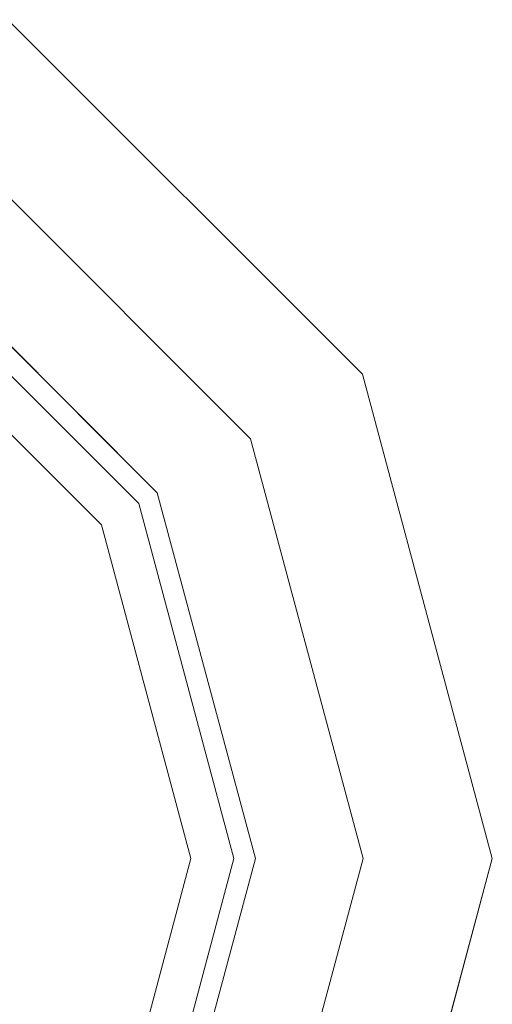
# Model space of a CAD drawing. Units: inches. Extents: x 375 to 1122, y 27 to 1069.
# Tile 45 of 155: x 715.392 to 718.094, y 302.255 to 307.886. Entities that reach past the tile are written whole.
import ezdxf

# ---------------------------------------------------------------- set-up
doc = ezdxf.new("R2010")
doc.units = ezdxf.units.IN
doc.layers.add('Furniture', color=30, linetype='Continuous', lineweight=18)

# ---------------------------------------------------------------- blocks, each defined once
blk = doc.blocks.new('A$C403C54AD')
at = {"linetype": 'ByBlock'}
for points, invisible_edges in [([(1.0802, 0.82864, -0.00874), (1.0802, 0.81017, -0.00874), (1.02018, 0.79408, -0.00874), (1.01094, 0.81008, -0.00874)], 5), ([(1.0802, 0.79478, -0.02259), (1.0802, 0.82864, -0.01335), (1.01094, 0.81008, -0.01335), (1.02787, 0.78075, -0.02259)], 5), ([(1.14947, 0.81008, -0.00874), (1.14023, 0.79408, -0.00874), (1.0802, 0.81017, -0.00874), (1.0802, 0.82864, -0.00874)], 5), ([(1.13254, 0.78075, -0.02259), (1.14947, 0.81008, -0.01335), (1.0802, 0.82864, -0.01335), (1.0802, 0.79478, -0.02259)], 5), ([(1.01094, 0.81008, -0.00874), (1.02018, 0.79408, -0.00874), (0.97623, 0.75014, -0.00874), (0.96024, 0.75938, -0.00874)], 5), ([(1.02787, 0.78075, -0.02259), (1.01094, 0.81008, -0.01335), (0.96024, 0.75938, -0.01335), (0.98956, 0.74244, -0.02259)], 5), ([(1.0802, 0.81017, -0.00874), (1.0802, 0.7917, -0.01489), (1.02941, 0.77809, -0.01489), (1.02018, 0.79408, -0.00874)], 5), ([(1.14023, 0.79408, -0.00874), (1.131, 0.77809, -0.01489), (1.0802, 0.7917, -0.01489), (1.0802, 0.81017, -0.00874)], 5), ([(1.02018, 0.79408, -0.00874), (1.02941, 0.77809, -0.01489), (0.99223, 0.74091, -0.01489), (0.97623, 0.75014, -0.00874)], 5), ([(1.0802, 0.78554, -0.03183), (1.0802, 0.79478, -0.02259), (1.02787, 0.78075, -0.02259), (1.03249, 0.77276, -0.03183)], 5), ([(1.12792, 0.77276, -0.03183), (1.13254, 0.78075, -0.02259), (1.0802, 0.79478, -0.02259), (1.0802, 0.78554, -0.03183)], 5), ([(1.0802, 0.7917, -0.01489), (1.0802, 0.69011, -0.01489), (1.0802, 0.69011, -0.01489), (1.02941, 0.77809, -0.01489)], 5), ([(1.131, 0.77809, -0.01489), (1.0802, 0.69011, -0.01489), (1.0802, 0.69011, -0.01489), (1.0802, 0.7917, -0.01489)], 5), ([(1.03249, 0.77276, -0.03183), (1.02787, 0.78075, -0.02259), (0.98956, 0.74244, -0.02259), (0.99756, 0.73783, -0.03183)], 1), ([(1.02941, 0.77809, -0.01489), (1.0802, 0.69011, -0.01489), (1.0802, 0.69011, -0.01489), (0.99223, 0.74091, -0.01489)], 5), ([(1.16818, 0.74091, -0.01489), (1.0802, 0.69011, -0.01489), (1.0802, 0.69011, -0.01489), (1.131, 0.77809, -0.01489)], 5)]:
    blk.add_3dface(points, dxfattribs=dict(at, invisible_edges=invisible_edges))
for points in [[(1.0802, 0.82864, -0.01335), (1.0802, 0.82864, -0.00874), (1.01094, 0.81008, -0.00874), (1.01094, 0.81008, -0.01335)], [(1.14947, 0.81008, -0.01335), (1.14947, 0.81008, -0.00874), (1.0802, 0.82864, -0.00874), (1.0802, 0.82864, -0.01335)], [(1.01094, 0.81008, -0.01335), (1.01094, 0.81008, -0.00874), (0.96024, 0.75938, -0.00874), (0.96024, 0.75938, -0.01335)]]:
    blk.add_3dface(points, dxfattribs=at)

msp = doc.modelspace()

# ---------------------------------------------------------------- block references
at = {"layer": 'Furniture', "xscale": 39.9918517141215, "yscale": 39.9918517141215, "zscale": 39.9918517141215, "rotation": 270}
msp.add_blockref('A$C403C54AD', (684.9549, 346.2875, 0.024), dxfattribs=at)

doc.saveas('drawing.dxf')
